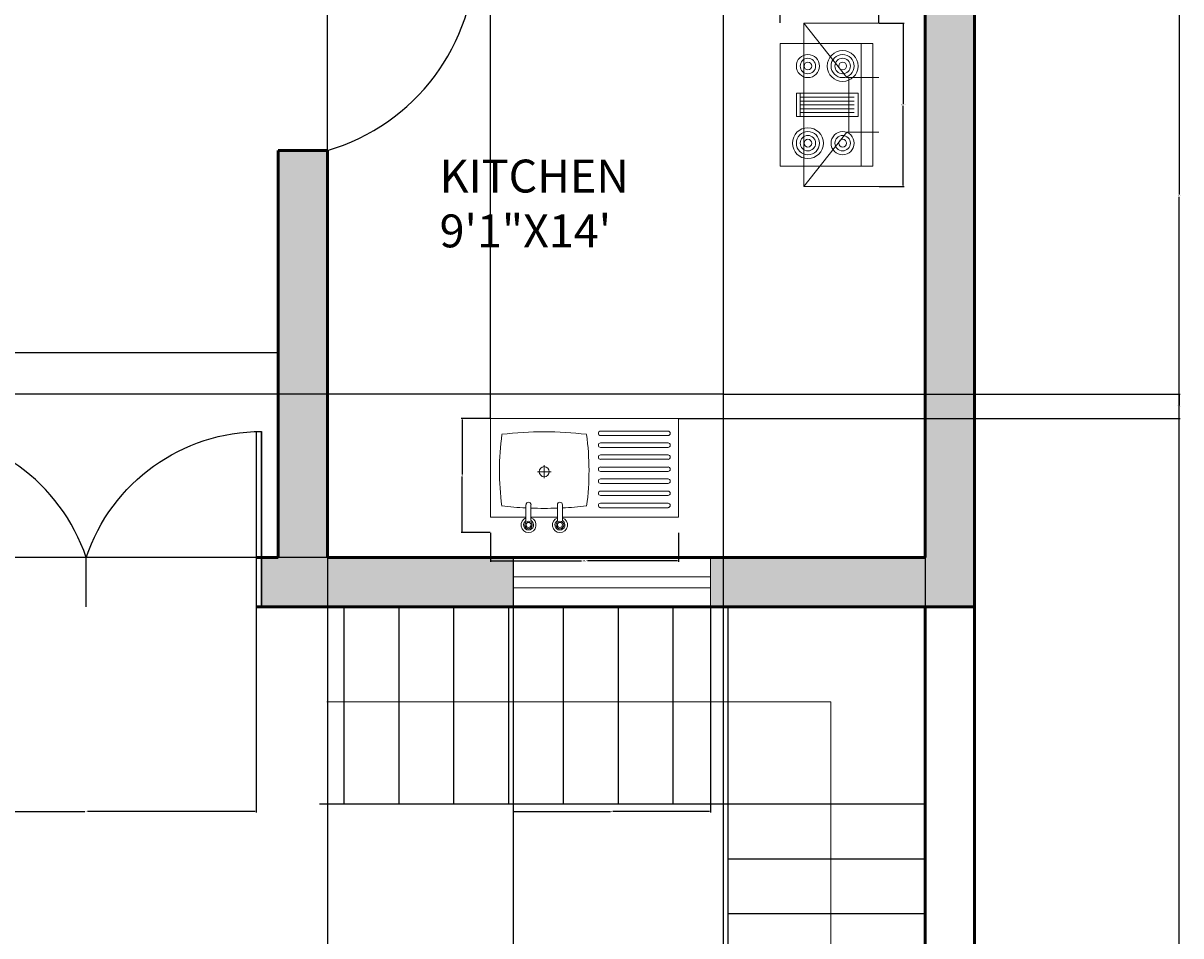
# Model space of a CAD drawing. Units: inches. Extents: x 383 to 970, y 275 to 1088.
# Tile 9 of 11: x 759 to 970, y 546 to 713. Entities that reach past the tile are written whole.
import ezdxf

# ---------------------------------------------------------------- set-up
doc = ezdxf.new("R2010")
doc.units = ezdxf.units.IN
doc.header["$MEASUREMENT"] = 0
for name, color, linetype, lineweight in [('A-ANNO-DIMS', 2, 'Continuous', 18), ('A-ANNO-SYMB', 7, 'Continuous', 18), ('A-AREA-IDEN', 7, 'Continuous', 18), ('A-DOOR', 3, 'Continuous', 25), ('A-EQPM', 8, 'Continuous', 18), ('A-FLOR-CASE', 8, 'Continuous', 25), ('A-FLOR-FIXT', 8, 'Continuous', 18), ('A-FLOR-STRS', 7, 'Continuous', 25), ('A-GLAZ', 4, 'Continuous', 18), ('A-WALL', 7, 'Continuous', 50)]:
    doc.layers.add(name, color=color, linetype=linetype, lineweight=lineweight)
doc.layers.add('A-WALL-PATT', color=251, linetype='Continuous', lineweight=13, true_color=0x636466)
doc.styles.get("Standard").update_dxf_attribs({"font": 'arial.ttf'})
doc.dimstyles.get("Standard").update_dxf_attribs({"dimtxt": 0.18, "dimasz": 0.18, "dimexe": 0.18, "dimexo": 0.0625, "dimgap": 0.09, "dimtad": 0, "dimtih": 1, "dimtoh": 1, "dimdec": 4, "dimzin": 0, "dimdsep": 46, "dimtxsty": 'Standard', "dimcen": 0.09, "dimadec": 0, "dimazin": 0, "dimtfac": 1, "dimtdec": 4, "dimtofl": 0, "dimtmove": 0, "dimatfit": 3, "dimfxl": 1, "dimtolj": 1, "dimtzin": 0, "dimarcsym": 0})

# ---------------------------------------------------------------- blocks, each defined once
blk = doc.blocks.new('chimmne')
for p, q in [((17.89, 6.07), (-18.11, 6.07)), ((-18.11, 6.07), (-18.11, -10.43)), ((-6.16, -3.43), (-18.11, 6.07)), ((5.94, -3.43), (17.89, 6.07)), ((17.89, 6.07), (17.89, -10.43)), ((-6.16, -3.43), (-6.16, -10.43)), ((5.94, -3.82), (-6.16, -3.82)), ((5.94, -3.43), (5.94, -10.43))]:
    blk.add_line(p, q)
for points in [[(-13.61, -9.12), (-13.61, 11.28), (13.39, 11.28), (13.39, -9.12)], [(-2.66, -5.87), (-2.66, 7.73), (2.44, 7.73), (2.44, -5.87)]]:
    blk.add_lwpolyline(points, close=True)
for points in [[(-2.66, 6.88), (2.44, 6.88)], [(-1.81, 6.88), (-1.81, -5.02)], [(-0.96, -5.02), (-0.96, 6.88)], [(-0.11, 6.88), (-0.11, -5.02)], [(0.74, -5.02), (0.74, 6.88)], [(1.59, 6.88), (1.59, -5.02)], [(13.39, -6.57), (-13.61, -6.57)]]:
    blk.add_lwpolyline(points)
for centre, radius in [((-8.55, 5.18), 3.4), ((-8.55, 5.18), 2.55), ((8.44, 5.18), 2.55), ((-8.55, 5.18), 1.7), ((-8.55, 5.18), 0.85), ((8.44, 5.18), 1.7), ((8.44, 5.18), 0.85), ((-8.55, -2.47), 2.55), ((8.44, -2.47), 3.4), ((8.44, -2.47), 2.55), ((-8.55, -2.47), 1.7), ((-8.55, -2.47), 0.85), ((8.44, -2.47), 1.7), ((8.44, -2.47), 0.85)]:
    blk.add_circle(centre, radius)
blk = doc.blocks.new('A$C799204C7')
for p, q in [((0, 34.2), (17.99, 34.2)), ((0, 0), (0, 34.2)), ((17.99, 13.08), (17.99, 34.2)), ((2.32, 20.01), (2.32, 32.27)), ((3.13, 20.01), (3.13, 32.27)), ((4.48, 20.01), (4.48, 32.27)), ((5.29, 20.01), (5.29, 32.27)), ((6.64, 20.01), (6.64, 32.27)), ((7.45, 20.01), (7.45, 32.27)), ((8.85, 20.01), (8.85, 32.27)), ((9.66, 20.01), (9.66, 32.27)), ((11.01, 20.01), (11.01, 32.27)), ((11.82, 20.01), (11.82, 32.27)), ((13.22, 20.01), (13.22, 32.27)), ((14.03, 20.01), (14.03, 32.27)), ((15.42, 20.01), (15.42, 32.27)), ((16.24, 20.01), (16.24, 32.27)), ((18.59, 13.08), (15.71, 13.08)), ((9.73, 11), (9.73, 8.54)), ((15.71, 12.17), (18.59, 12.17)), ((17.99, 7.36), (17.99, 12.17)), ((8.52, 9.77), (10.9, 9.77)), ((18.59, 7.36), (15.71, 7.36)), ((15.71, 6.45), (18.59, 6.45)), ((17.99, 0), (17.99, 6.45)), ((0, 0), (17.99, 0))]:
    blk.add_line(p, q)
for centre, radius in [((19.38, 12.62), 0.684), ((19.38, 12.62), 0.456), ((9.7, 9.77), 0.916), ((19.38, 6.91), 0.684), ((19.38, 6.91), 0.456)]:
    blk.add_circle(centre, radius)
for centre, radius, start, end in [((2.72, 32.27), 0.407, 0, 180), ((4.88, 32.27), 0.407, 0, 180), ((7.05, 32.27), 0.407, 0, 180), ((9.25, 32.27), 0.407, 0, 180), ((11.42, 32.27), 0.407, 0, 180), ((13.62, 32.27), 0.407, 0, 180), ((15.83, 32.27), 0.407, 0, 180), ((2.72, 20.01), 0.407, 180, 0), ((4.88, 20.01), 0.407, 180, 0), ((7.05, 20.01), 0.407, 180, 0), ((9.25, 20.01), 0.407, 180, 0), ((11.42, 20.01), 0.407, 180, 0), ((13.62, 20.01), 0.407, 180, 0), ((15.83, 20.01), 0.407, 180, 0), ((67.33, 9.77), 64.88, 173.1952, 186.8048), ((9.53, -30.19), 48.1, 82.3437, 97.8966), ((-48.51, 9.77), 64.88, 2.9208, 6.8048), ((15.71, 12.62), 0.456, 90, 270), ((19.38, 12.62), 1.37, 199.6514, 160.3603), ((19.38, 12.62), 0.911, 210.3431, 149.7554), ((-48.51, 9.77), 64.88, 357.8723, 2.115), ((15.71, 6.91), 0.456, 90, 270), ((-48.51, 9.77), 64.88, 353.1952, 357.0665), ((19.38, 6.91), 1.37, 199.6514, 160.3603), ((19.38, 6.91), 0.911, 210.3431, 149.7554), ((9.53, 49.73), 48.1, 262.1034, 277.6563)]:
    blk.add_arc(centre, radius, start, end)
blk = doc.blocks.new('DOOR-LEAF-36IN')
for p, q in [((0, 0), (0, 36)), ((1, 36), (1, 0)), ((0, 0), (1, 0))]:
    blk.add_line(p, q)
blk.add_arc((0, -1.5), 37.5, 16.2602, 90)
blk = doc.blocks.new('DOOR-LEAF-32IN')
for p, q in [((32, 32), (31, 32)), ((31, 0), (31, 32)), ((32, 32), (32, 0))]:
    blk.add_line(p, q)
blk.add_arc((32, 33.76), 33.76, 198.5866, 270)
blk = doc.blocks.new('*D33')
at = {"layer": 'A-ANNO-DIMS', "color": 0, "lineweight": -2, "transparency": 16777216}
for p, q in [((914.86, 712.6), (919.45, 712.6)), ((919.27, 712.42), (919.27, 697.88)), ((919.27, 682.97), (919.27, 697.51)), ((914.86, 682.79), (919.45, 682.79))]:
    blk.add_line(p, q, dxfattribs=at)
at = {"layer": 'A-ANNO-DIMS', "color": 0, "transparency": 16777216}
for points in [[(919.24, 712.42), (919.3, 712.42), (919.27, 712.6)], [(919.24, 682.97), (919.3, 682.97), (919.27, 682.79)]]:
    blk.add_solid(points, dxfattribs=at)
at = {"layer": 'Defpoints', "color": 0, "transparency": 16777216}
for p in [(914.8, 712.6), (919.27, 712.6), (914.8, 682.79)]:
    blk.add_point(p, dxfattribs=at)
at = {"layer": 'A-ANNO-DIMS', "color": 0, "transparency": 16777216, "insert": (919.27, 697.7), "char_height": 0.18, "attachment_point": 5}
blk.add_mtext('\\A1;HOB 30', dxfattribs=at)
blk = doc.blocks.new('*D34')
at = {"layer": 'A-ANNO-DIMS', "color": 0, "lineweight": -2, "transparency": 16777216}
for p, q in [((896.83, 712.66), (896.83, 717.25)), ((897.01, 717.07), (905.6, 717.07)), ((914.62, 717.07), (906.02, 717.07)), ((914.8, 712.66), (914.8, 717.25))]:
    blk.add_line(p, q, dxfattribs=at)
at = {"layer": 'A-ANNO-DIMS', "color": 0, "transparency": 16777216}
for points in [[(897.01, 717.1), (897.01, 717.04), (896.83, 717.07)], [(914.62, 717.1), (914.62, 717.04), (914.8, 717.07)]]:
    blk.add_solid(points, dxfattribs=at)
at = {"layer": 'Defpoints', "color": 0, "transparency": 16777216}
for p in [(896.83, 717.07), (896.83, 712.6), (914.8, 712.6)]:
    blk.add_point(p, dxfattribs=at)
at = {"layer": 'A-ANNO-DIMS', "color": 0, "transparency": 16777216, "insert": (905.81, 717.07), "char_height": 0.18, "attachment_point": 5}
blk.add_mtext('\\A1;18', dxfattribs=at)
blk = doc.blocks.new('*D35')
at = {"layer": 'A-ANNO-DIMS', "color": 0, "lineweight": -2, "transparency": 16777216}
for p, q in [((843.98, 619.65), (843.98, 614.38)), ((878.29, 619.65), (878.29, 614.38)), ((844.16, 614.56), (860.59, 614.56)), ((878.11, 614.56), (861.69, 614.56))]:
    blk.add_line(p, q, dxfattribs=at)
at = {"layer": 'A-ANNO-DIMS', "color": 0, "transparency": 16777216}
for points in [[(844.16, 614.59), (844.16, 614.53), (843.98, 614.56)], [(878.11, 614.59), (878.11, 614.53), (878.29, 614.56)]]:
    blk.add_solid(points, dxfattribs=at)
at = {"layer": 'Defpoints', "color": 0, "transparency": 16777216}
for p in [(843.98, 619.71), (878.29, 619.71), (878.29, 614.56)]:
    blk.add_point(p, dxfattribs=at)
at = {"layer": 'A-ANNO-DIMS', "color": 0, "transparency": 16777216, "insert": (861.14, 614.56), "char_height": 0.18, "attachment_point": 5}
blk.add_mtext('\\A1;SINK 34', dxfattribs=at)
blk = doc.blocks.new('*D36')
at = {"layer": 'A-ANNO-DIMS', "color": 0, "lineweight": -2, "transparency": 16777216}
for p, q in [((843.92, 640.52), (838.66, 640.52)), ((838.84, 640.34), (838.84, 630.3)), ((838.84, 619.89), (838.84, 629.94)), ((843.92, 619.71), (838.66, 619.71))]:
    blk.add_line(p, q, dxfattribs=at)
at = {"layer": 'A-ANNO-DIMS', "color": 0, "transparency": 16777216}
for points in [[(838.81, 640.34), (838.87, 640.34), (838.84, 640.52)], [(838.81, 619.89), (838.87, 619.89), (838.84, 619.71)]]:
    blk.add_solid(points, dxfattribs=at)
at = {"layer": 'Defpoints', "color": 0, "transparency": 16777216}
for p in [(843.98, 640.52), (838.84, 619.71), (843.98, 619.71)]:
    blk.add_point(p, dxfattribs=at)
at = {"layer": 'A-ANNO-DIMS', "color": 0, "transparency": 16777216, "insert": (838.84, 630.12), "char_height": 0.18, "attachment_point": 5}
blk.add_mtext('\\A1;21', dxfattribs=at)
blk = doc.blocks.new('*D38')
at = {"layer": 'A-ANNO-DIMS', "color": 0, "lineweight": -2, "transparency": 16777216}
for p, q in [((932.3, 1050.14), (969.77, 1050.14)), ((969.59, 1049.96), (969.59, 681.32)), ((969.59, 312.32), (969.59, 680.95)), ((932.3, 312.14), (969.77, 312.14))]:
    blk.add_line(p, q, dxfattribs=at)
at = {"layer": 'A-ANNO-DIMS', "color": 0, "transparency": 16777216}
for points in [[(969.56, 1049.96), (969.62, 1049.96), (969.59, 1050.14)], [(969.56, 312.32), (969.62, 312.32), (969.59, 312.14)]]:
    blk.add_solid(points, dxfattribs=at)
at = {"layer": 'Defpoints', "color": 0, "transparency": 16777216}
for p in [(932.24, 1050.14), (969.59, 1050.14), (932.24, 312.14)]:
    blk.add_point(p, dxfattribs=at)
at = {"layer": 'A-ANNO-DIMS', "color": 0, "transparency": 16777216, "insert": (969.59, 681.14), "char_height": 0.18, "attachment_point": 5}
blk.add_mtext('\\A1;738', dxfattribs=at)
blk = doc.blocks.new('*D54')
at = {"layer": 'A-ANNO-DIMS', "color": 0, "lineweight": -2, "transparency": 16777216}
for p, q in [((814.18, 644.96), (382.71, 644.96)), ((382.89, 644.78), (382.89, 630.23)), ((382.89, 615.32), (382.89, 629.86)), ((814.18, 615.14), (382.71, 615.14))]:
    blk.add_line(p, q, dxfattribs=at)
at = {"layer": 'A-ANNO-DIMS', "color": 0, "transparency": 16777216}
for points in [[(382.86, 644.78), (382.92, 644.78), (382.89, 644.96)], [(382.86, 615.32), (382.92, 615.32), (382.89, 615.14)]]:
    blk.add_solid(points, dxfattribs=at)
at = {"layer": 'Defpoints', "color": 0, "transparency": 16777216}
for p in [(382.89, 644.96), (814.24, 644.96), (814.24, 615.14)]:
    blk.add_point(p, dxfattribs=at)
at = {"layer": 'A-ANNO-DIMS', "color": 0, "transparency": 16777216, "insert": (382.89, 630.05), "char_height": 0.18, "attachment_point": 5}
blk.add_mtext('\\A1;29.82', dxfattribs=at)
blk = doc.blocks.new('*D55')
at = {"layer": 'A-ANNO-DIMS', "color": 0, "lineweight": -2, "transparency": 16777216}
for p, q in [((886.41, 644.89), (886.41, 274.61)), ((923.24, 615.07), (923.24, 274.61)), ((886.59, 274.79), (904.36, 274.79)), ((923.06, 274.79), (905.29, 274.79))]:
    blk.add_line(p, q, dxfattribs=at)
at = {"layer": 'A-ANNO-DIMS', "color": 0, "transparency": 16777216}
for points in [[(886.59, 274.82), (886.59, 274.76), (886.41, 274.79)], [(923.06, 274.82), (923.06, 274.76), (923.24, 274.79)]]:
    blk.add_solid(points, dxfattribs=at)
at = {"layer": 'Defpoints', "color": 0, "transparency": 16777216}
for p in [(886.41, 644.96), (923.24, 615.14), (923.24, 274.79)]:
    blk.add_point(p, dxfattribs=at)
at = {"layer": 'A-ANNO-DIMS', "color": 0, "transparency": 16777216, "insert": (904.82, 274.79), "char_height": 0.18, "attachment_point": 5}
blk.add_mtext('\\A1;36.834', dxfattribs=at)
blk = doc.blocks.new('*D57')
at = {"layer": 'A-ANNO-DIMS', "color": 0, "lineweight": -2, "transparency": 16777216}
for p, q in [((814.24, 615.07), (814.24, 274.61)), ((848.09, 615.07), (848.09, 274.61)), ((814.42, 274.79), (830.77, 274.79)), ((847.91, 274.79), (831.56, 274.79))]:
    blk.add_line(p, q, dxfattribs=at)
at = {"layer": 'A-ANNO-DIMS', "color": 0, "transparency": 16777216}
for points in [[(814.42, 274.82), (814.42, 274.76), (814.24, 274.79)], [(847.91, 274.82), (847.91, 274.76), (848.09, 274.79)]]:
    blk.add_solid(points, dxfattribs=at)
at = {"layer": 'Defpoints', "color": 0, "transparency": 16777216}
for p in [(814.24, 615.14), (848.09, 615.14), (848.09, 274.79)]:
    blk.add_point(p, dxfattribs=at)
at = {"layer": 'A-ANNO-DIMS', "color": 0, "transparency": 16777216, "insert": (831.16, 274.79), "char_height": 0.18, "attachment_point": 5}
blk.add_mtext('\\A1;33.85', dxfattribs=at)
blk = doc.blocks.new('*D58')
at = {"layer": 'A-ANNO-DIMS', "color": 0, "lineweight": -2, "transparency": 16777216}
for p, q in [((848.09, 606.07), (848.09, 568.61)), ((884.09, 606.07), (884.09, 568.61)), ((848.27, 568.79), (865.87, 568.79)), ((883.91, 568.79), (866.31, 568.79))]:
    blk.add_line(p, q, dxfattribs=at)
at = {"layer": 'A-ANNO-DIMS', "color": 0, "transparency": 16777216}
for points in [[(848.27, 568.82), (848.27, 568.76), (848.09, 568.79)], [(883.91, 568.82), (883.91, 568.76), (884.09, 568.79)]]:
    blk.add_solid(points, dxfattribs=at)
at = {"layer": 'Defpoints', "color": 0, "transparency": 16777216}
for p in [(848.09, 606.14), (884.09, 606.14), (848.09, 568.79)]:
    blk.add_point(p, dxfattribs=at)
at = {"layer": 'A-ANNO-DIMS', "color": 0, "transparency": 16777216, "insert": (866.09, 568.79), "char_height": 0.18, "attachment_point": 5}
blk.add_mtext('\\A1;36', dxfattribs=at)
blk = doc.blocks.new('*D59')
at = {"layer": 'A-ANNO-DIMS', "color": 0, "lineweight": -2, "transparency": 16777216}
for p, q in [((814.24, 645.02), (814.24, 1087.67)), ((814.42, 1087.49), (828.65, 1087.49)), ((843.8, 1087.49), (829.58, 1087.49)), ((843.98, 640.59), (843.98, 1087.67))]:
    blk.add_line(p, q, dxfattribs=at)
at = {"layer": 'A-ANNO-DIMS', "color": 0, "transparency": 16777216}
for points in [[(814.42, 1087.52), (814.42, 1087.46), (814.24, 1087.49)], [(843.8, 1087.52), (843.8, 1087.46), (843.98, 1087.49)]]:
    blk.add_solid(points, dxfattribs=at)
at = {"layer": 'Defpoints', "color": 0, "transparency": 16777216}
for p in [(814.24, 1087.49), (814.24, 644.96), (843.98, 640.52)]:
    blk.add_point(p, dxfattribs=at)
at = {"layer": 'A-ANNO-DIMS', "color": 0, "transparency": 16777216, "insert": (829.11, 1087.49), "char_height": 0.18, "attachment_point": 5}
blk.add_mtext('\\A1;29.744', dxfattribs=at)
blk = doc.blocks.new('*D67')
at = {"layer": 'A-ANNO-DIMS', "color": 0, "lineweight": -2, "transparency": 16777216}
for p, q in [((498.24, 615.2), (498.24, 652.67)), ((498.42, 652.49), (651.45, 652.49)), ((805.06, 652.49), (652.03, 652.49)), ((805.24, 615.2), (805.24, 652.67))]:
    blk.add_line(p, q, dxfattribs=at)
at = {"layer": 'A-ANNO-DIMS', "color": 0, "transparency": 16777216}
for points in [[(498.42, 652.52), (498.42, 652.46), (498.24, 652.49)], [(805.06, 652.52), (805.06, 652.46), (805.24, 652.49)]]:
    blk.add_solid(points, dxfattribs=at)
at = {"layer": 'Defpoints', "color": 0, "transparency": 16777216}
for p in [(805.24, 652.49), (498.24, 615.14), (805.24, 615.14)]:
    blk.add_point(p, dxfattribs=at)
at = {"layer": 'A-ANNO-DIMS', "color": 0, "transparency": 16777216, "insert": (651.74, 652.49), "char_height": 0.18, "attachment_point": 5}
blk.add_mtext('\\A1;307', dxfattribs=at)
blk = doc.blocks.new('*D68')
at = {"layer": 'A-ANNO-DIMS', "color": 0, "lineweight": -2, "transparency": 16777216}
for p, q in [((739.24, 606.07), (739.24, 568.61)), ((801.24, 606.07), (801.24, 568.61)), ((739.42, 568.79), (770.02, 568.79)), ((801.06, 568.79), (770.46, 568.79))]:
    blk.add_line(p, q, dxfattribs=at)
at = {"layer": 'A-ANNO-DIMS', "color": 0, "transparency": 16777216}
for points in [[(739.42, 568.82), (739.42, 568.76), (739.24, 568.79)], [(801.06, 568.82), (801.06, 568.76), (801.24, 568.79)]]:
    blk.add_solid(points, dxfattribs=at)
at = {"layer": 'Defpoints', "color": 0, "transparency": 16777216}
for p in [(739.24, 606.14), (801.24, 606.14), (739.24, 568.79)]:
    blk.add_point(p, dxfattribs=at)
at = {"layer": 'A-ANNO-DIMS', "color": 0, "transparency": 16777216, "insert": (770.24, 568.79), "char_height": 0.18, "attachment_point": 5}
blk.add_mtext('\\A1;62', dxfattribs=at)
blk = doc.blocks.new('*D69')
at = {"layer": 'A-ANNO-DIMS', "color": 0, "lineweight": -2, "transparency": 16777216}
for p, q in [((886.47, 644.96), (969.77, 644.96)), ((969.59, 644.78), (969.59, 642.92)), ((969.59, 640.7), (969.59, 642.56)), ((878.36, 640.52), (969.77, 640.52))]:
    blk.add_line(p, q, dxfattribs=at)
at = {"layer": 'A-ANNO-DIMS', "color": 0, "transparency": 16777216}
for points in [[(969.56, 644.78), (969.62, 644.78), (969.59, 644.96)], [(969.56, 640.7), (969.62, 640.7), (969.59, 640.52)]]:
    blk.add_solid(points, dxfattribs=at)
at = {"layer": 'Defpoints', "color": 0, "transparency": 16777216}
for p in [(886.41, 644.96), (969.59, 644.96), (878.29, 640.52)]:
    blk.add_point(p, dxfattribs=at)
at = {"layer": 'A-ANNO-DIMS', "color": 0, "transparency": 16777216, "insert": (969.59, 642.74), "char_height": 0.18, "attachment_point": 5}
blk.add_mtext('\\A1;4.433', dxfattribs=at)

msp = doc.modelspace()

# ---------------------------------------------------------------- hatches: boundary and pattern name
at = {"layer": 'A-WALL-PATT'}
h = msp.add_hatch(color=256, dxfattribs=at)
h.dxf.hatch_style = 1
h.paths.add_polyline_path([(651.24, 321.1365), (651.24, 417.1365), (735.24, 417.1365), (735.24, 491.9233), (726.24, 491.9233), (726.24, 426.1365), (582.24, 426.1365), (582.24, 606.1365), (687.24, 606.1365), (687.24, 615.1365), (573.24, 615.1365), (573.24, 546.1365), (570.24, 546.1365), (570.24, 537.1365), (573.24, 537.1365), (573.24, 414.1365), (582.24, 414.1365), (582.24, 417.1365), (642.24, 417.1365), (642.24, 321.1365), (621.6203, 321.1365), (621.6203, 312.1365), (651.24, 312.1365)], flags=17)
h.paths.add_polyline_path([(597.6203, 321.1365), (582.24, 321.1365), (582.24, 390.1365), (573.24, 390.1365), (573.24, 321.1365), (570.24, 321.1365), (570.24, 312.1365), (573.24, 312.1365), (597.6203, 312.1365)], flags=16)
h.paths.add_polyline_path([(534.24, 321.1365), (500.8868, 321.1365), (500.8868, 312.1365), (534.24, 312.1365)], flags=17)
h.paths.add_polyline_path([(735.24, 606.1365), (738.24, 606.1365), (738.24, 615.1365), (723.24, 615.1365), (723.24, 606.1365), (726.24, 606.1365), (726.24, 551.9233), (735.24, 551.9233)], flags=17)
h.paths.add_polyline_path([(848.0899, 615.1365), (814.24, 615.1365), (814.24, 689.38), (805.24, 689.38), (805.24, 615.1365), (802.24, 615.1365), (802.24, 606.1365), (848.0899, 606.1365)], flags=17)
h.paths.add_polyline_path([(530.24, 615.1365), (498.24, 615.1365), (498.24, 646.5351), (489.24, 646.5351), (489.24, 615.1365), (466.771, 615.1365), (466.771, 606.1365), (521.24, 606.1365), (521.24, 603.1365), (530.24, 603.1365), (530.24, 606.1365)], flags=17)
h.paths.add_polyline_path([(498.24, 744.1365), (489.24, 744.1365), (489.24, 706.5351), (498.24, 706.5351)], flags=17)
h.paths.add_polyline_path([(715.24, 792.1365), (598.24, 792.1365), (598.24, 972.1365), (636.5058, 972.1365), (636.5058, 981.1365), (589.24, 981.1365), (589.24, 972.1365), (589.24, 792.1365), (586.24, 792.1365), (586.24, 783.1365), (589.24, 783.1365), (715.24, 783.1365)], flags=17)
h.paths.add_polyline_path([(763.24, 981.1365), (696.5058, 981.1365), (696.5058, 972.1365), (754.24, 972.1365), (754.24, 792.1365), (751.24, 792.1365), (751.24, 783.1365), (754.24, 783.1365), (764.24, 783.1365), (764.24, 792.1365), (763.24, 792.1365)], flags=17)
h.paths.add_polyline_path([(815.24, 1001.9492), (806.24, 1001.9492), (806.24, 972.1365), (818.24, 972.1365), (818.24, 981.1365), (815.24, 981.1365)], flags=17)
h.paths.add_polyline_path([(546.24, 1004.0336), (537.24, 1004.0336), (537.24, 981.1365), (534.24, 981.1365), (534.24, 972.1365), (537.24, 972.1365), (546.24, 972.1365), (546.24, 981.1365)], flags=17)
h.paths.add_polyline_path([(884.0899, 606.1365), (932.24, 606.1365), (932.24, 1050.1365), (420.24, 1050.1365), (420.24, 312.1365), (440.8868, 312.1365), (440.8868, 321.1365), (429.24, 321.1365), (429.24, 537.1365), (538.24, 537.1365), (538.24, 546.1365), (530.24, 546.1365), (530.24, 579.1365), (521.24, 579.1365), (521.24, 546.1365), (429.24, 546.1365), (429.24, 606.1365), (442.771, 606.1365), (442.771, 615.1365), (429.24, 615.1365), (429.24, 783.1365), (489.24, 783.1365), (489.24, 780.1365), (498.24, 780.1365), (498.24, 783.1365), (550.24, 783.1365), (550.24, 792.1365), (429.24, 792.1365), (429.24, 972.1365), (510.24, 972.1365), (510.24, 981.1365), (429.24, 981.1365), (429.24, 1041.1365), (537.24, 1041.1365), (537.24, 1028.0336), (546.24, 1028.0336), (546.24, 1041.1365), (806.24, 1041.1365), (806.24, 1025.9492), (815.24, 1025.9492), (815.24, 1041.1365), (923.24, 1041.1365), (923.24, 981.1365), (842.24, 981.1365), (842.24, 972.1365), (923.24, 972.1365), (923.24, 792.1365), (800.24, 792.1365), (800.24, 783.1365), (805.24, 783.1365), (805.24, 725.38), (814.24, 725.38), (814.24, 783.1365), (923.24, 783.1365), (923.24, 615.1365), (884.0899, 615.1365)])

# ---------------------------------------------------------------- linework, layer by layer
at = {"layer": 'A-ANNO-SYMB'}
for p, q in [((814.1456, 588.7988), (906.0568, 588.7988)), ((906.0568, 588.7988), (906.0568, 535.5591))]:
    msp.add_line(p, q, dxfattribs=at)
at = {"layer": 'A-DOOR'}
for p, q in [((802.24, 638.1365), (802.24, 606.1365)), ((770.24, 606.1365), (770.24, 615.1365)), ((801.24, 606.1365), (802.24, 606.1365))]:
    msp.add_line(p, q, dxfattribs=at)
at = {"layer": 'A-FLOR-CASE'}
for p, q in [((886.4057, 753.7583), (886.4057, 644.9565)), ((886.4057, 644.9565), (814.24, 644.9565))]:
    msp.add_line(p, q, dxfattribs=at)
at = {"layer": 'A-FLOR-STRS'}
for p, q in [((817.24, 606.1365), (817.24, 570.1365)), ((827.24, 606.1365), (827.24, 570.1365)), ((837.24, 606.1365), (837.24, 570.1365)), ((847.24, 606.1365), (847.24, 570.1365)), ((857.24, 606.1365), (857.24, 570.1365)), ((867.24, 606.1365), (867.24, 570.1365)), ((877.24, 606.1365), (877.24, 570.1365)), ((923.24, 606.1365), (887.24, 606.1365)), ((887.24, 606.1365), (887.24, 475.2293)), ((923.24, 606.1365), (923.24, 570.1365)), ((923.24, 570.1365), (812.8124, 570.1365)), ((923.24, 560.1365), (887.24, 560.1365)), ((923.24, 550.1365), (887.24, 550.1365))]:
    msp.add_line(p, q, dxfattribs=at)
at = {"layer": 'A-GLAZ'}
for p, q in [((848.0899, 615.1365), (848.0899, 606.1365)), ((884.0899, 615.1365), (848.0899, 615.1365)), ((884.0899, 606.1365), (884.0899, 615.1365)), ((884.0899, 611.6365), (848.0899, 611.6365)), ((848.0899, 609.6365), (884.0899, 609.6365)), ((848.0899, 606.1365), (884.0899, 606.1365))]:
    msp.add_line(p, q, dxfattribs=at)
at = {"layer": 'A-WALL'}
for p, q in [((932.24, 1050.1365), (932.24, 312.1365)), ((923.24, 783.1365), (923.24, 615.1365)), ((805.24, 689.38), (814.24, 689.38)), ((805.24, 689.38), (805.24, 615.1365)), ((814.24, 689.38), (814.24, 615.1365)), ((801.24, 615.1365), (805.24, 615.1365)), ((814.24, 615.1365), (923.24, 615.1365)), ((801.24, 606.1365), (923.24, 606.1365)), ((923.24, 606.1365), (923.24, 312.1365)), ((923.24, 606.1365), (932.24, 606.1365))]:
    msp.add_line(p, q, dxfattribs=at)

# ---------------------------------------------------------------- block references
at = {"layer": 'A-DOOR'}
for name, p, rotation in [('DOOR-LEAF-36IN', (805.2396, 725.3801), 270), ('DOOR-LEAF-32IN', (770.2401, 638.137), 180)]:
    msp.add_blockref(name, p, dxfattribs=dict(at, rotation=rotation))
at = {"layer": 'A-DOOR', "extrusion": (0, 0, -1), "zscale": -1, "rotation": 180}
msp.add_blockref('DOOR-LEAF-32IN', (-770.24, 638.137), dxfattribs=at)
at = {"layer": 'A-EQPM', "xscale": 0.8280321260258986, "yscale": 0.8280321260258986, "zscale": 0.8280321260258986, "rotation": 90}
msp.add_blockref('chimmne', (906.1647, 697.7893), dxfattribs=at)
at = {"layer": 'A-FLOR-FIXT', "xscale": 1.0032, "yscale": 1.0032, "zscale": 1.0032, "rotation": 270}
msp.add_blockref('A$C799204C7', (843.9841, 640.5231), dxfattribs=at)

# ---------------------------------------------------------------- texts
at = {"layer": 'A-AREA-IDEN', "insert": (834.6936, 687.7114), "char_height": 6, "attachment_point": 1}
msp.add_mtext_dynamic_manual_height_columns('KITCHEN\\P9\'1"X14\'', width=46.129192, gutter_width=30, heights=[0], dxfattribs=at)

# ---------------------------------------------------------------- dimensions: what is measured, and where the dimension line sits
at = {"layer": 'A-ANNO-DIMS'}
for base, p1, p2, override, picture, middle in [((814.24, 1087.4865), (843.9841, 640.5231), (814.24, 644.9565), {"dimdec": 3, "dimlfac": 1, "dimrnd": 0, "dimzin": 0, "dimdsep": 46, "dimlunit": 2}, '*D59', (829.1121, 1087.4865)), ((805.24, 652.4865), (498.24, 615.1365), (805.24, 615.1365), {"dimdec": 0, "dimlfac": 1, "dimrnd": 0, "dimzin": 0, "dimdsep": 46, "dimlunit": 2}, '*D67', (651.74, 652.4865)), ((923.24, 274.7865), (886.4057, 644.9565), (923.24, 615.1365), {"dimdec": 3, "dimlfac": 1, "dimrnd": 0, "dimzin": 0, "dimdsep": 46, "dimlunit": 2}, '*D55', (904.8229, 274.7865)), ((848.0899, 274.7865), (814.24, 615.1365), (848.0899, 615.1365), {"dimdec": 2, "dimlfac": 1, "dimrnd": 0, "dimzin": 0, "dimdsep": 46, "dimlunit": 2}, '*D57', (831.165, 274.7865))]:
    dim = msp.add_linear_dim(base=base, p1=p1, p2=p2, dimstyle='Standard', override=override, dxfattribs=at)
    dim.commit()
    dim.dimension.update_dxf_attribs({"geometry": picture, "text_midpoint": middle})
for base, p1, p2, angle, override, picture, middle in [((969.59, 1050.1365), (932.24, 312.1365), (932.24, 1050.1365), 90, {"dimdec": 0, "dimlfac": 1, "dimrnd": 0, "dimzin": 0, "dimdsep": 46, "dimlunit": 2}, '*D38', (969.59, 681.1365)), ((896.8275, 717.0724), (914.8009, 712.601), (896.8275, 712.601), 180, {"dimdec": 0, "dimlfac": 1, "dimrnd": 0, "dimzin": 0, "dimdsep": 46, "dimlunit": 2}, '*D34', (905.8142, 717.0724)), ((382.89, 644.9565), (814.24, 615.1365), (814.24, 644.9565), 90, {"dimdec": 2, "dimlfac": 1, "dimrnd": 0, "dimzin": 0, "dimdsep": 46, "dimlunit": 2}, '*D54', (382.89, 630.0465)), ((969.59, 644.9565), (878.2935, 640.5231), (886.4057, 644.9565), 90, {"dimdec": 3, "dimlfac": 1, "dimrnd": 0, "dimzin": 0, "dimdsep": 46, "dimlunit": 2}, '*D69', (969.59, 642.7398)), ((838.8377, 619.7091), (843.9841, 640.5231), (843.9841, 619.7091), 270, {"dimdec": 0, "dimlfac": 1, "dimrnd": 0, "dimzin": 0, "dimdsep": 46, "dimlunit": 2}, '*D36', (838.8377, 630.1161)), ((739.24, 568.7865), (801.24, 606.1365), (739.24, 606.1365), 180, {"dimdec": 0, "dimlfac": 1, "dimrnd": 0, "dimzin": 0, "dimdsep": 46, "dimlunit": 2}, '*D68', (770.24, 568.7865)), ((848.0899, 568.7865), (884.0899, 606.1365), (848.0899, 606.1365), 180, {"dimdec": 0, "dimlfac": 1, "dimrnd": 0, "dimzin": 0, "dimdsep": 46, "dimlunit": 2}, '*D58', (866.0899, 568.7865))]:
    dim = msp.add_linear_dim(base=base, p1=p1, p2=p2, angle=angle, dimstyle='Standard', override=override, dxfattribs=at)
    dim.commit()
    dim.dimension.update_dxf_attribs({"geometry": picture, "text_midpoint": middle})
dim = msp.add_linear_dim(base=(919.2723, 712.601), p1=(914.8009, 682.7918), p2=(914.8009, 712.601), angle=90, text='HOB <>', dimstyle='Standard', override={"dimdec": 0, "dimlfac": 1, "dimrnd": 0, "dimzin": 0, "dimdsep": 46, "dimlunit": 2}, dxfattribs=at)
dim.commit()
dim.dimension.update_dxf_attribs({"geometry": '*D33', "text_midpoint": (919.2723, 697.6964)})
dim = msp.add_linear_dim(base=(878.2935, 614.5627), p1=(843.9841, 619.7091), p2=(878.2935, 619.7091), text='SINK <>', dimstyle='Standard', override={"dimdec": 0, "dimlfac": 1, "dimrnd": 0, "dimzin": 0, "dimdsep": 46, "dimlunit": 2}, dxfattribs=at)
dim.commit()
dim.dimension.update_dxf_attribs({"geometry": '*D35', "text_midpoint": (861.1388, 614.5627)})

doc.saveas('drawing.dxf')
